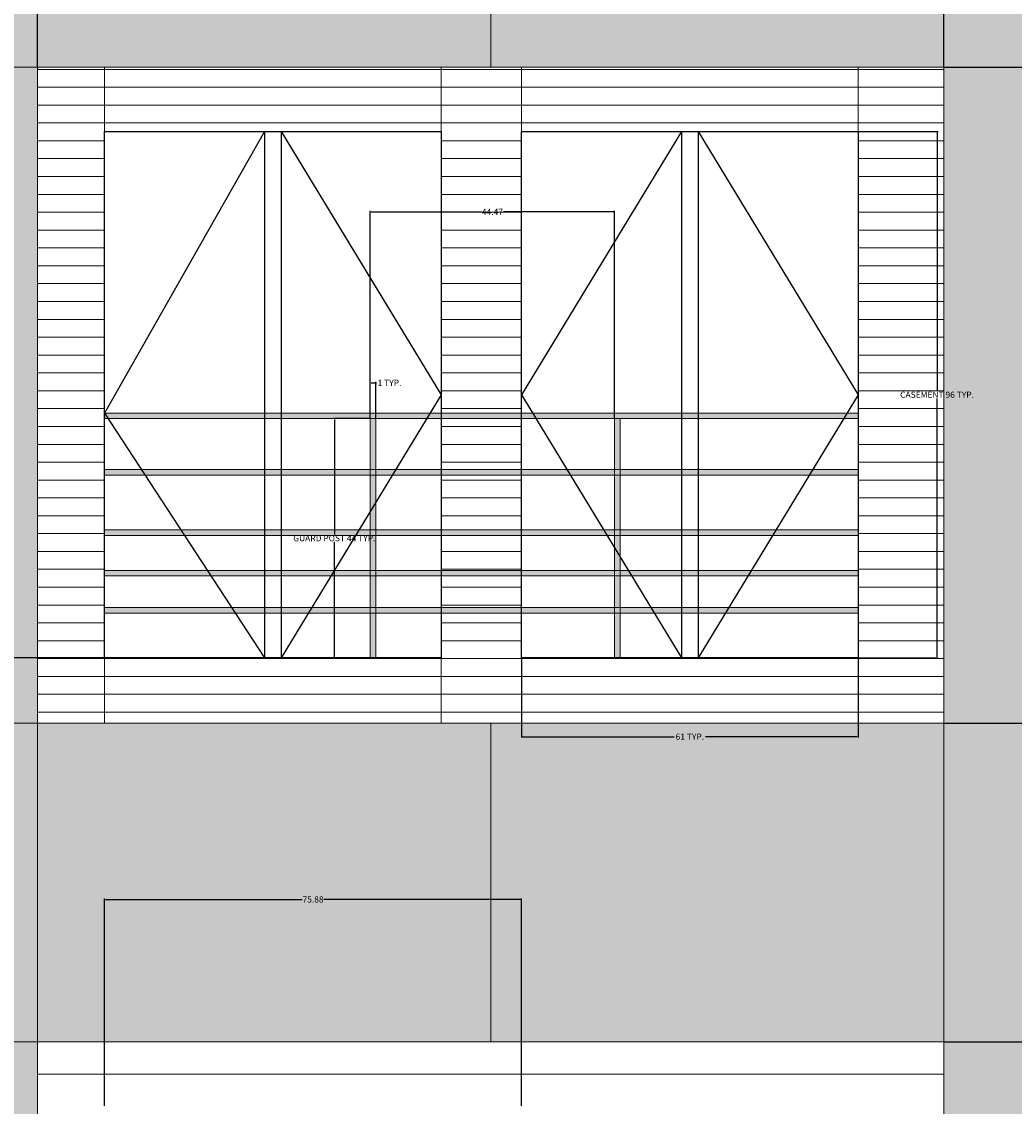
# Model space of a CAD drawing. Units: inches. Extents: x 8 to 634, y 41 to 867.
# Tile 6 of 21: x 117 to 297, y 380 to 577. Entities that reach past the tile are written whole.
import ezdxf

# ---------------------------------------------------------------- set-up
doc = ezdxf.new("R2010")
doc.units = ezdxf.units.IN
doc.header["$MEASUREMENT"] = 0
for name, color, linetype, lineweight in [('A-ANNO-DIMS', 2, 'Continuous', 18), ('A-FLOR-HRAL', 7, 'Continuous', 18), ('A-FLOR-HRAL-PATT', 252, 'Continuous', 9), ('A-GLAZ', 4, 'Continuous', 25), ('A-WALL-PANL', 7, 'Continuous', 18), ('A-WALL-PATT', 8, 'Continuous', 9)]:
    doc.layers.add(name, color=color, linetype=linetype, lineweight=lineweight)
doc.styles.get("Standard").update_dxf_attribs({"font": 'arial.ttf'})
doc.dimstyles.get("Standard").update_dxf_attribs({"dimtxt": 1.125, "dimasz": 0.18, "dimexe": 0.18, "dimexo": 0.0625, "dimgap": 0.09, "dimtad": 0, "dimtih": 1, "dimtoh": 1, "dimdec": 4, "dimzin": 0, "dimdsep": 46, "dimlunit": 4, "dimtxsty": 'Standard', "dimcen": 0.09, "dimadec": 0, "dimazin": 0, "dimtfac": 1, "dimtdec": 4, "dimtofl": 0, "dimtmove": 0, "dimatfit": 3, "dimfxl": 1, "dimtolj": 1, "dimtzin": 0, "dimarcsym": 0})

# ---------------------------------------------------------------- blocks, each defined once
blk = doc.blocks.new('WIN-CASEMENT-FRAME')
for p, q in [((29.12, 95.77), (29.12, 0)), ((32.12, 95.77), (32.12, 0))]:
    blk.add_line(p, q)
blk.add_lwpolyline([(0, 95.77), (61.23, 95.77), (61.23, 0), (0, 0)], close=True)
blk = doc.blocks.new('GUARD-POST')
for p, q in [((0, 42.52), (0, 43.52)), ((1, 42.52), (1, 43.52)), ((0, 42.52), (0, 0)), ((1, 42.52), (1, 0))]:
    blk.add_line(p, q)
blk = doc.blocks.new('*D13')
at = {"layer": 'A-ANNO-DIMS', "color": 0, "lineweight": -2, "transparency": 16777216}
for p, q in [((269.05, 557.42), (283.53, 557.42)), ((283.35, 557.24), (283.35, 510.21)), ((283.35, 461.83), (283.35, 508.86)), ((269.05, 461.65), (283.53, 461.65))]:
    blk.add_line(p, q, dxfattribs=at)
at = {"layer": 'A-ANNO-DIMS', "color": 0, "transparency": 16777216}
for points in [[(283.32, 557.24), (283.38, 557.24), (283.35, 557.42)], [(283.32, 461.83), (283.38, 461.83), (283.35, 461.65)]]:
    blk.add_solid(points, dxfattribs=at)
at = {"layer": 'Defpoints', "color": 0, "transparency": 16777216}
for p in [(268.99, 557.42), (283.35, 557.42), (268.99, 461.65)]:
    blk.add_point(p, dxfattribs=at)
at = {"layer": 'A-ANNO-DIMS', "color": 0, "transparency": 16777216, "insert": (283.35, 509.53), "char_height": 1.125, "attachment_point": 5}
blk.add_mtext('\\A1;CASEMENT 96 TYP.', dxfattribs=at)
blk = doc.blocks.new('*D14')
at = {"layer": 'A-ANNO-DIMS', "color": 0, "lineweight": -2, "transparency": 16777216}
for p, q in [((207.75, 461.59), (207.75, 447.11)), ((268.99, 461.59), (268.99, 447.11)), ((207.93, 447.29), (235.54, 447.29)), ((268.81, 447.29), (241.2, 447.29))]:
    blk.add_line(p, q, dxfattribs=at)
at = {"layer": 'A-ANNO-DIMS', "color": 0, "transparency": 16777216}
for points in [[(207.93, 447.32), (207.93, 447.26), (207.75, 447.29)], [(268.81, 447.32), (268.81, 447.26), (268.99, 447.29)]]:
    blk.add_solid(points, dxfattribs=at)
at = {"layer": 'Defpoints', "color": 0, "transparency": 16777216}
for p in [(207.75, 461.65), (268.99, 461.65), (268.99, 447.29)]:
    blk.add_point(p, dxfattribs=at)
at = {"layer": 'A-ANNO-DIMS', "color": 0, "transparency": 16777216, "insert": (238.37, 447.29), "char_height": 1.125, "attachment_point": 5}
blk.add_mtext('\\A1;61 TYP.', dxfattribs=at)
blk = doc.blocks.new('*D15')
at = {"layer": 'A-ANNO-DIMS', "color": 0, "lineweight": -2, "transparency": 16777216}
for p, q in [((180.15, 505.18), (173.51, 505.18)), ((173.69, 505), (173.69, 484.09)), ((173.69, 461.83), (173.69, 482.74)), ((180.15, 461.65), (173.51, 461.65))]:
    blk.add_line(p, q, dxfattribs=at)
at = {"layer": 'A-ANNO-DIMS', "color": 0, "transparency": 16777216}
for points in [[(173.66, 505), (173.72, 505), (173.69, 505.18)], [(173.66, 461.83), (173.72, 461.83), (173.69, 461.65)]]:
    blk.add_solid(points, dxfattribs=at)
at = {"layer": 'Defpoints', "color": 0, "transparency": 16777216}
for p in [(173.69, 505.18), (180.21, 505.18), (180.21, 461.65)]:
    blk.add_point(p, dxfattribs=at)
at = {"layer": 'A-ANNO-DIMS', "color": 0, "transparency": 16777216, "insert": (173.69, 483.41), "char_height": 1.125, "attachment_point": 5}
blk.add_mtext('\\A1;GUARD POST 44 TYP.', dxfattribs=at)
blk = doc.blocks.new('*D16')
at = {"layer": 'A-ANNO-DIMS', "color": 0, "lineweight": -2, "transparency": 16777216}
for p, q in [((180.21, 505.24), (180.21, 511.88)), ((180.39, 511.7), (181.03, 511.7)), ((181.21, 505.24), (181.21, 511.88)), ((181.21, 511.7), (181.39, 511.7))]:
    blk.add_line(p, q, dxfattribs=at)
at = {"layer": 'A-ANNO-DIMS', "color": 0, "transparency": 16777216}
for points in [[(180.39, 511.73), (180.39, 511.67), (180.21, 511.7)], [(181.03, 511.73), (181.03, 511.67), (181.21, 511.7)]]:
    blk.add_solid(points, dxfattribs=at)
at = {"layer": 'Defpoints', "color": 0, "transparency": 16777216}
for p in [(181.21, 511.7), (180.21, 505.18), (181.21, 505.18)]:
    blk.add_point(p, dxfattribs=at)
at = {"layer": 'A-ANNO-DIMS', "color": 0, "transparency": 16777216, "insert": (183.73, 511.7), "char_height": 1.125, "attachment_point": 5}
blk.add_mtext('\\A1;1 TYP.', dxfattribs=at)
blk = doc.blocks.new('*D20')
at = {"layer": 'A-ANNO-DIMS', "color": 0, "lineweight": -2, "transparency": 16777216}
for p, q in [((144.29, 828.98), (9.51, 828.98)), ((9.69, 828.8), (9.69, 454.93)), ((9.69, 79.74), (9.69, 453.6)), ((47.28, 79.56), (9.51, 79.56))]:
    blk.add_line(p, q, dxfattribs=at)
at = {"layer": 'A-ANNO-DIMS', "color": 0, "transparency": 16777216}
for points in [[(9.66, 828.8), (9.72, 828.8), (9.69, 828.98)], [(9.66, 79.74), (9.72, 79.74), (9.69, 79.56)]]:
    blk.add_solid(points, dxfattribs=at)
at = {"layer": 'Defpoints', "color": 0, "transparency": 16777216}
for p in [(9.69, 828.98), (144.36, 828.98), (47.34, 79.56)]:
    blk.add_point(p, dxfattribs=at)
at = {"layer": 'A-ANNO-DIMS', "color": 0, "transparency": 16777216, "insert": (9.69, 454.27), "char_height": 1.125, "attachment_point": 5}
blk.add_mtext('\\A1;749.4', dxfattribs=at)
blk = doc.blocks.new('*D41')
at = {"layer": 'A-ANNO-DIMS', "color": 0, "lineweight": -2, "transparency": 16777216}
for p, q in [((131.88, 380.07), (131.88, 417.84)), ((132.06, 417.66), (167.83, 417.66)), ((207.57, 417.66), (171.8, 417.66)), ((207.75, 380.07), (207.75, 417.84))]:
    blk.add_line(p, q, dxfattribs=at)
at = {"layer": 'A-ANNO-DIMS', "color": 0, "transparency": 16777216}
for points in [[(132.06, 417.69), (132.06, 417.63), (131.88, 417.66)], [(207.57, 417.69), (207.57, 417.63), (207.75, 417.66)]]:
    blk.add_solid(points, dxfattribs=at)
at = {"layer": 'Defpoints', "color": 0, "transparency": 16777216}
for p in [(207.75, 417.66), (131.88, 380.01), (207.75, 380.01)]:
    blk.add_point(p, dxfattribs=at)
at = {"layer": 'A-ANNO-DIMS', "color": 0, "transparency": 16777216, "insert": (169.82, 417.66), "char_height": 1.125, "attachment_point": 5}
blk.add_mtext('\\A1;75.88', dxfattribs=at)
blk = doc.blocks.new('*D43')
at = {"layer": 'A-ANNO-DIMS', "color": 0, "lineweight": -2, "transparency": 16777216}
for p, q in [((131.81, 461.65), (94.05, 461.65)), ((94.23, 461.47), (94.23, 373.6)), ((94.23, 284.42), (94.23, 372.29)), ((131.81, 284.24), (94.05, 284.24))]:
    blk.add_line(p, q, dxfattribs=at)
at = {"layer": 'A-ANNO-DIMS', "color": 0, "transparency": 16777216}
for points in [[(94.2, 461.47), (94.26, 461.47), (94.23, 461.65)], [(94.2, 284.42), (94.26, 284.42), (94.23, 284.24)]]:
    blk.add_solid(points, dxfattribs=at)
at = {"layer": 'Defpoints', "color": 0, "transparency": 16777216}
for p in [(94.23, 461.65), (131.88, 461.65), (131.88, 284.24)]:
    blk.add_point(p, dxfattribs=at)
at = {"layer": 'A-ANNO-DIMS', "color": 0, "transparency": 16777216, "insert": (94.23, 372.95), "char_height": 1.125, "attachment_point": 5}
blk.add_mtext('\\A1;177.4', dxfattribs=at)
blk = doc.blocks.new('*D57')
at = {"layer": 'A-ANNO-DIMS', "color": 0, "lineweight": -2, "transparency": 16777216}
for p, q in [((119.71, 569.23), (119.71, 607)), ((119.89, 606.82), (200.22, 606.82)), ((284.43, 606.82), (204.09, 606.82)), ((284.61, 569.23), (284.61, 607))]:
    blk.add_line(p, q, dxfattribs=at)
at = {"layer": 'A-ANNO-DIMS', "color": 0, "transparency": 16777216}
for points in [[(119.89, 606.85), (119.89, 606.79), (119.71, 606.82)], [(284.43, 606.85), (284.43, 606.79), (284.61, 606.82)]]:
    blk.add_solid(points, dxfattribs=at)
at = {"layer": 'Defpoints', "color": 0, "transparency": 16777216}
for p in [(284.61, 606.82), (119.71, 569.17), (284.61, 569.17)]:
    blk.add_point(p, dxfattribs=at)
at = {"layer": 'A-ANNO-DIMS', "color": 0, "transparency": 16777216, "insert": (202.16, 606.82), "char_height": 1.125, "attachment_point": 5}
blk.add_mtext('\\A1;164.9', dxfattribs=at)
blk = doc.blocks.new('*D58')
at = {"layer": 'A-ANNO-DIMS', "color": 0, "lineweight": -2, "transparency": 16777216}
for p, q in [((47.34, 569.23), (47.34, 607)), ((47.52, 606.82), (81.54, 606.82)), ((119.53, 606.82), (85.51, 606.82)), ((119.71, 569.23), (119.71, 607))]:
    blk.add_line(p, q, dxfattribs=at)
at = {"layer": 'A-ANNO-DIMS', "color": 0, "transparency": 16777216}
for points in [[(47.52, 606.85), (47.52, 606.79), (47.34, 606.82)], [(119.53, 606.85), (119.53, 606.79), (119.71, 606.82)]]:
    blk.add_solid(points, dxfattribs=at)
at = {"layer": 'Defpoints', "color": 0, "transparency": 16777216}
for p in [(119.71, 606.82), (47.34, 569.17), (119.71, 569.17)]:
    blk.add_point(p, dxfattribs=at)
at = {"layer": 'A-ANNO-DIMS', "color": 0, "transparency": 16777216, "insert": (83.52, 606.82), "char_height": 1.125, "attachment_point": 5}
blk.add_mtext('\\A1;72.37', dxfattribs=at)
blk = doc.blocks.new('*D59')
at = {"layer": 'A-ANNO-DIMS', "color": 0, "lineweight": -2, "transparency": 16777216}
for p, q in [((284.67, 449.75), (322.44, 449.75)), ((322.26, 449.57), (322.26, 421.42)), ((322.26, 391.94), (322.26, 420.09)), ((284.67, 391.76), (322.44, 391.76))]:
    blk.add_line(p, q, dxfattribs=at)
at = {"layer": 'A-ANNO-DIMS', "color": 0, "transparency": 16777216}
for points in [[(322.23, 449.57), (322.29, 449.57), (322.26, 449.75)], [(322.23, 391.94), (322.29, 391.94), (322.26, 391.76)]]:
    blk.add_solid(points, dxfattribs=at)
at = {"layer": 'Defpoints', "color": 0, "transparency": 16777216}
for p in [(284.61, 449.75), (284.61, 391.76), (322.26, 391.76)]:
    blk.add_point(p, dxfattribs=at)
at = {"layer": 'A-ANNO-DIMS', "color": 0, "transparency": 16777216, "insert": (322.26, 420.76), "char_height": 1.125, "attachment_point": 5}
blk.add_mtext('\\A1;57.99', dxfattribs=at)
blk = doc.blocks.new('*D60')
at = {"layer": 'A-ANNO-DIMS', "color": 0, "lineweight": -2, "transparency": 16777216}
for p, q in [((284.67, 569.17), (322.44, 569.17)), ((322.26, 568.99), (322.26, 510.13)), ((322.26, 449.93), (322.26, 508.8)), ((284.67, 449.75), (322.44, 449.75))]:
    blk.add_line(p, q, dxfattribs=at)
at = {"layer": 'A-ANNO-DIMS', "color": 0, "transparency": 16777216}
for points in [[(322.23, 568.99), (322.29, 568.99), (322.26, 569.17)], [(322.23, 449.93), (322.29, 449.93), (322.26, 449.75)]]:
    blk.add_solid(points, dxfattribs=at)
at = {"layer": 'Defpoints', "color": 0, "transparency": 16777216}
for p in [(284.61, 569.17), (284.61, 449.75), (322.26, 449.75)]:
    blk.add_point(p, dxfattribs=at)
at = {"layer": 'A-ANNO-DIMS', "color": 0, "transparency": 16777216, "insert": (322.26, 509.46), "char_height": 1.125, "attachment_point": 5}
blk.add_mtext('\\A1;119.42', dxfattribs=at)
blk = doc.blocks.new('*D62')
at = {"layer": 'A-ANNO-DIMS', "color": 0, "lineweight": -2, "transparency": 16777216}
for p, q in [((180.21, 505.24), (180.21, 543.01)), ((224.68, 505.24), (224.68, 543.01)), ((180.39, 542.83), (200.44, 542.83)), ((224.5, 542.83), (204.46, 542.83))]:
    blk.add_line(p, q, dxfattribs=at)
at = {"layer": 'A-ANNO-DIMS', "color": 0, "transparency": 16777216}
for points in [[(180.39, 542.86), (180.39, 542.8), (180.21, 542.83)], [(224.5, 542.86), (224.5, 542.8), (224.68, 542.83)]]:
    blk.add_solid(points, dxfattribs=at)
at = {"layer": 'Defpoints', "color": 0, "transparency": 16777216}
for p in [(224.68, 542.83), (180.21, 505.18), (224.68, 505.18)]:
    blk.add_point(p, dxfattribs=at)
at = {"layer": 'A-ANNO-DIMS', "color": 0, "transparency": 16777216, "insert": (202.45, 542.83), "char_height": 1.125, "attachment_point": 5}
blk.add_mtext('\\A1;44.47', dxfattribs=at)

msp = doc.modelspace()

# ---------------------------------------------------------------- hatches: boundary and pattern name
at = {"layer": 'A-FLOR-HRAL-PATT', "transparency": 33554681}
h = msp.add_hatch(color=256, dxfattribs=at)
h.dxf.hatch_style = 1
h.paths.add_polyline_path([(266.9465, 506.1755), (239.872, 506.1755), (239.872, 505.1755), (266.3384, 505.1755)])
h.paths.add_polyline_path([(236.872, 506.1755), (209.7974, 506.1755), (210.4055, 505.1755), (236.872, 505.1755)])
h.paths.add_polyline_path([(239.872, 506.1755), (236.872, 506.1755), (236.872, 505.1755), (239.872, 505.1755)])
h.paths.add_polyline_path([(268.9893, 506.1755), (266.9465, 506.1755), (266.3384, 505.1755), (268.9893, 505.1755)])
h.paths.add_polyline_path([(268.9893, 495.8921), (260.6935, 495.8921), (260.0854, 494.8921), (268.9893, 494.8921)])
h.paths.add_polyline_path([(260.6935, 495.8921), (239.872, 495.8921), (239.872, 494.8921), (260.0854, 494.8921)])
h.paths.add_polyline_path([(239.872, 495.8921), (236.872, 495.8921), (236.872, 494.8921), (239.872, 494.8921)])
h.paths.add_polyline_path([(236.872, 495.8921), (225.6812, 495.8921), (225.6812, 494.8921), (236.872, 494.8921)])
h.paths.add_polyline_path([(191.0689, 506.1755), (163.9944, 506.1755), (163.9944, 505.1755), (190.4608, 505.1755)])
h.paths.add_polyline_path([(193.1116, 506.1755), (191.0689, 506.1755), (190.4608, 505.1755), (193.1116, 505.1755)])
h.paths.add_polyline_path([(209.7974, 506.1755), (207.7547, 506.1755), (207.7547, 505.1755), (210.4055, 505.1755)])
h.paths.add_polyline_path([(207.7547, 506.1755), (193.1116, 506.1755), (193.1116, 505.1755), (207.7547, 505.1755)])
h.paths.add_polyline_path([(207.7547, 495.8921), (193.1116, 495.8921), (193.1116, 494.8921), (207.7547, 494.8921)])
h.paths.add_polyline_path([(216.0505, 495.8921), (207.7547, 495.8921), (207.7547, 494.8921), (216.6586, 494.8921)])
h.paths.add_polyline_path([(224.6812, 495.8921), (216.0505, 495.8921), (216.6586, 494.8921), (224.6812, 494.8921)])
h.paths.add_polyline_path([(225.6812, 495.8921), (224.6812, 495.8921), (224.6812, 494.8921), (225.6812, 494.8921)])
h.paths.add_polyline_path([(222.7266, 484.913), (207.7547, 484.913), (207.7547, 483.913), (223.3347, 483.913)])
h.paths.add_polyline_path([(207.7547, 484.913), (193.1116, 484.913), (193.1116, 483.913), (207.7547, 483.913)])
h.paths.add_polyline_path([(225.6812, 484.913), (224.6812, 484.913), (224.6812, 483.913), (225.6812, 483.913)])
h.paths.add_polyline_path([(224.6812, 484.913), (222.7266, 484.913), (223.3347, 483.913), (224.6812, 483.913)])
h.paths.add_polyline_path([(236.872, 484.913), (225.6812, 484.913), (225.6812, 483.913), (236.872, 483.913)])
h.paths.add_polyline_path([(239.872, 484.913), (236.872, 484.913), (236.872, 483.913), (239.872, 483.913)])
h.paths.add_polyline_path([(254.0173, 484.913), (239.872, 484.913), (239.872, 483.913), (253.4093, 483.913)])
h.paths.add_polyline_path([(268.9893, 484.913), (254.0173, 484.913), (253.4093, 483.913), (268.9893, 483.913)])
h.paths.add_polyline_path([(268.9893, 477.5606), (249.5465, 477.5606), (248.9384, 476.5606), (268.9893, 476.5606)])
h.paths.add_polyline_path([(249.5465, 477.5606), (239.872, 477.5606), (239.872, 476.5606), (248.9384, 476.5606)])
h.paths.add_polyline_path([(245.427, 470.7859), (239.872, 470.7859), (239.872, 469.7859), (244.8189, 469.7859)])
h.paths.add_polyline_path([(268.9893, 470.7859), (245.427, 470.7859), (244.8189, 469.7859), (268.9893, 469.7859)])
h.paths.add_polyline_path([(239.872, 470.7859), (236.872, 470.7859), (236.872, 469.7859), (239.872, 469.7859)])
h.paths.add_polyline_path([(239.872, 477.5606), (236.872, 477.5606), (236.872, 476.5606), (239.872, 476.5606)])
h.paths.add_polyline_path([(236.872, 477.5606), (227.1975, 477.5606), (227.8055, 476.5606), (236.872, 476.5606)])
h.paths.add_polyline_path([(236.872, 470.7859), (231.317, 470.7859), (231.9251, 469.7859), (236.872, 469.7859)])
h.paths.add_polyline_path([(231.317, 470.7859), (225.6812, 470.7859), (225.6812, 469.7859), (231.9251, 469.7859)])
h.paths.add_polyline_path([(225.6812, 470.7859), (224.6812, 470.7859), (224.6812, 469.7859), (225.6812, 469.7859)])
h.paths.add_polyline_path([(225.6812, 469.7859), (224.6812, 469.7859), (224.6812, 461.6505), (225.6812, 461.6505)])
h.paths.add_polyline_path([(225.6812, 476.5606), (224.6812, 476.5606), (224.6812, 470.7859), (225.6812, 470.7859)])
h.paths.add_polyline_path([(225.6812, 477.5606), (224.6812, 477.5606), (224.6812, 476.5606), (225.6812, 476.5606)])
h.paths.add_polyline_path([(225.6812, 480.0542), (224.6812, 481.6987), (224.6812, 477.5606), (225.6812, 477.5606)])
h.paths.add_polyline_path([(227.1975, 477.5606), (225.6812, 477.5606), (225.6812, 476.5606), (227.8055, 476.5606)])
h.paths.add_polyline_path([(224.6812, 477.5606), (207.7547, 477.5606), (207.7547, 476.5606), (224.6812, 476.5606)])
h.paths.add_polyline_path([(224.6812, 470.7859), (207.7547, 470.7859), (207.7547, 469.7859), (224.6812, 469.7859)])
h.paths.add_polyline_path([(225.6812, 483.913), (224.6812, 483.913), (224.6812, 481.6987), (225.6812, 480.0542)])
h.paths.add_polyline_path([(207.7547, 477.5606), (193.1116, 477.5606), (193.1116, 476.5606), (207.7547, 476.5606)])
h.paths.add_polyline_path([(207.7547, 470.7859), (193.1116, 470.7859), (193.1116, 469.7859), (207.7547, 469.7859)])
h.paths.add_polyline_path([(193.1116, 470.7859), (181.2144, 470.7859), (181.2144, 469.7859), (193.1116, 469.7859)])
h.paths.add_polyline_path([(193.1116, 477.5606), (181.2144, 477.5606), (181.2144, 476.5606), (193.1116, 476.5606)])
h.paths.add_polyline_path([(181.2144, 470.7859), (131.8771, 470.7859), (131.8771, 469.7859), (181.2144, 469.7859)])
h = msp.add_hatch(color=256, dxfattribs=at)
h.dxf.hatch_style = 1
h.paths.add_polyline_path([(180.2144, 477.5606), (173.6689, 477.5606), (173.0608, 476.5606), (180.2144, 476.5606)])
h.paths.add_polyline_path([(181.2144, 483.913), (180.2144, 483.913), (180.2144, 477.5606), (181.2144, 477.5606)])
h.paths.add_polyline_path([(181.2144, 476.5606), (180.2144, 476.5606), (180.2144, 470.7859), (181.2144, 470.7859)])
h.paths.add_polyline_path([(181.2144, 477.5606), (180.2144, 477.5606), (180.2144, 476.5606), (181.2144, 476.5606)])
h.paths.add_polyline_path([(181.2144, 469.7859), (180.2144, 469.7859), (180.2144, 461.6505), (181.2144, 461.6505)])
h.paths.add_polyline_path([(163.9944, 477.5606), (160.9944, 477.5606), (160.9944, 476.5606), (163.9944, 476.5606)])
h.paths.add_polyline_path([(173.6689, 477.5606), (163.9944, 477.5606), (163.9944, 476.5606), (173.0608, 476.5606)])
h.paths.add_polyline_path([(160.9944, 477.5606), (150.5899, 477.5606), (151.2439, 476.5606), (160.9944, 476.5606)])
h.paths.add_polyline_path([(150.5899, 477.5606), (131.8771, 477.5606), (131.8771, 476.5606), (151.2439, 476.5606)])
h.paths.add_polyline_path([(160.9944, 484.913), (145.7818, 484.913), (146.4357, 483.913), (160.9944, 483.913)])
h.paths.add_polyline_path([(145.7818, 484.913), (131.8771, 484.913), (131.8771, 483.913), (146.4357, 483.913)])
h.paths.add_polyline_path([(163.9944, 484.913), (160.9944, 484.913), (160.9944, 483.913), (163.9944, 483.913)])
h.paths.add_polyline_path([(178.1397, 484.913), (163.9944, 484.913), (163.9944, 483.913), (177.5316, 483.913)])
h.paths.add_polyline_path([(181.2144, 484.913), (180.2144, 484.913), (180.2144, 483.913), (181.2144, 483.913)])
h.paths.add_polyline_path([(181.2144, 489.9695), (180.2144, 488.3249), (180.2144, 484.913), (181.2144, 484.913)])
h.paths.add_polyline_path([(193.1116, 484.913), (181.2144, 484.913), (181.2144, 483.913), (193.1116, 483.913)])
h.paths.add_polyline_path([(180.2144, 484.913), (178.1397, 484.913), (177.5316, 483.913), (180.2144, 483.913)])
h.paths.add_polyline_path([(181.2144, 495.8921), (180.2144, 495.8921), (180.2144, 494.8921), (181.2144, 494.8921)])
h.paths.add_polyline_path([(181.2144, 494.8921), (180.2144, 494.8921), (180.2144, 488.3249), (181.2144, 489.9695)])
h.paths.add_polyline_path([(184.8158, 495.8921), (181.2144, 495.8921), (181.2144, 494.8921), (184.2078, 494.8921)])
h.paths.add_polyline_path([(193.1116, 495.8921), (184.8158, 495.8921), (184.2078, 494.8921), (193.1116, 494.8921)])
h.paths.add_polyline_path([(180.2144, 495.8921), (163.9944, 495.8921), (163.9944, 494.8921), (180.2144, 494.8921)])
h.paths.add_polyline_path([(163.9944, 495.8921), (160.9944, 495.8921), (160.9944, 494.8921), (163.9944, 494.8921)])
h.paths.add_polyline_path([(160.9944, 495.8921), (138.6019, 495.8921), (139.2559, 494.8921), (160.9944, 494.8921)])
h.paths.add_polyline_path([(138.6019, 495.8921), (131.8771, 495.8921), (131.8771, 494.8921), (139.2559, 494.8921)])
h.paths.add_polyline_path([(181.2144, 504.1755), (181.2144, 505.1755), (180.2144, 505.1755), (180.2144, 504.1755), (180.2144, 495.8921), (181.2144, 495.8921)])
h.paths.add_polyline_path([(225.6812, 494.8921), (224.6812, 494.8921), (224.6812, 484.913), (225.6812, 484.913)])
h.paths.add_polyline_path([(225.6812, 495.8921), (224.6812, 495.8921), (224.6812, 494.8921), (225.6812, 494.8921)])
h.paths.add_polyline_path([(225.6812, 504.1755), (225.6812, 505.1755), (224.6812, 505.1755), (224.6812, 504.1755), (224.6812, 495.8921), (225.6812, 495.8921)])
h.paths.add_polyline_path([(131.8771, 506.1755), (131.8771, 505.1755), (132.531, 505.1755)], flags=17)
h.paths.add_polyline_path([(193.1116, 506.1755), (131.8771, 506.1755), (132.531, 505.1755), (193.1116, 505.1755)])
at = {"layer": 'A-WALL-PATT', "transparency": 33554687}
h = msp.add_hatch(dxfattribs=at)
h.set_pattern_fill('AR-CONC', color=256, scale=3.2)
h.paths.add_polyline_path([(119.7065, 697.6655), (47.3401, 697.6655), (47.3401, 569.1705), (119.7065, 569.1705)])
h.paths.add_polyline_path([(202.1558, 697.6655), (119.7065, 697.6655), (119.7065, 569.1705), (202.1558, 569.1705)])
h.paths.add_polyline_path([(284.6051, 697.6655), (202.1558, 697.6655), (202.1558, 569.1705), (284.6051, 569.1705)])
h.paths.add_polyline_path([(119.7065, 569.1705), (47.3401, 569.1705), (47.3401, 523.5555), (47.3401, 449.7533), (119.7065, 449.7533)])
h.paths.add_polyline_path([(342.6544, 682.1444), (360.785, 697.6655), (284.6051, 697.6655), (284.6051, 569.1705), (342.6544, 569.1705)])
h.paths.add_polyline_path([(342.6544, 569.1705), (284.6051, 569.1705), (284.6051, 449.7533), (342.6544, 449.7533)])
h.paths.add_polyline_path([(418.2881, 691.978), (418.2881, 697.6655), (360.785, 697.6655), (360.785, 569.1705), (418.2881, 569.1705)])
h.paths.add_polyline_path([(418.2881, 569.1705), (360.785, 569.1705), (360.785, 523.5555), (360.785, 449.7533), (418.2881, 449.7533)])
h.paths.add_polyline_path([(594.3501, 697.6655), (539.0002, 697.6655), (539.0002, 691.978), (539.0002, 569.1705), (594.3501, 569.1705)])
h.paths.add_polyline_path([(594.3501, 523.5555), (594.3501, 569.1705), (539.0002, 569.1705), (539.0002, 451.6305), (594.3501, 451.6305)])
h.paths.add_polyline_path([(594.3501, 451.6305), (539.0002, 451.6305), (539.0002, 391.7598), (594.3501, 391.7598)])
h.paths.add_polyline_path([(594.3501, 391.7598), (539.0002, 391.7598), (539.0002, 276.166), (594.3501, 276.166)])
h.paths.add_polyline_path([(418.2881, 449.7533), (360.785, 449.7533), (360.785, 391.7598), (418.2881, 391.7598)])
h.paths.add_polyline_path([(342.6544, 449.7533), (284.6051, 449.7533), (284.6051, 391.7598), (342.6544, 391.7598)])
h.paths.add_polyline_path([(342.6544, 391.7598), (284.6051, 391.7598), (284.6051, 272.3426), (342.6544, 272.3426)])
h.paths.add_polyline_path([(418.2881, 391.7598), (360.785, 391.7598), (360.785, 272.3426), (418.2881, 272.3426)])
h.paths.add_polyline_path([(418.2881, 272.3426), (360.785, 272.3426), (360.785, 235.5555), (418.2881, 235.5555)])
h.paths.add_polyline_path([(342.6544, 272.3426), (284.6051, 272.3426), (284.6051, 235.5555), (295.0049, 235.5555), (342.6544, 235.5555)])
h.paths.add_polyline_path([(594.3501, 276.166), (539.0002, 276.166), (539.0002, 228.4951), (594.3501, 228.4951)])
h.paths.add_polyline_path([(594.3501, 228.4951), (539.0002, 228.4951), (539.0002, 91.5417), (594.3501, 91.5417)])
h.paths.add_polyline_path([(418.2881, 235.5555), (360.785, 235.5555), (360.785, 91.5417), (418.2881, 91.5417)])
h.paths.add_polyline_path([(284.6051, 272.3426), (119.7065, 272.3426), (119.7065, 235.5555), (284.6051, 235.5555)])
h.paths.add_polyline_path([(119.7065, 272.3426), (47.3401, 272.3426), (47.3401, 235.5555), (47.3401, 91.5555), (63.5448, 91.5555), (63.5448, 227.8036), (268.998, 227.8036), (268.998, 91.5555), (295.0049, 91.5555), (295.0049, 222.583), (271.9787, 222.583), (271.9787, 229.0481), (62.4019, 229.0481), (62.4019, 222.583), (61.1827, 222.583), (61.1827, 235.5555), (119.7065, 235.5555)])
h.paths.add_polyline_path([(119.7065, 391.7598), (47.3401, 391.7598), (47.3401, 379.5555), (47.3401, 272.3426), (119.7065, 272.3426)])
h.paths.add_polyline_path([(119.7065, 449.7533), (47.3401, 449.7533), (47.3401, 391.7598), (119.7065, 391.7598)])
h.paths.add_polyline_path([(202.1558, 449.7533), (119.7065, 449.7533), (119.7065, 391.7598), (202.1558, 391.7598)])
h.paths.add_polyline_path([(284.6051, 449.7533), (202.1558, 449.7533), (202.1558, 391.7598), (284.6051, 391.7598)])
at = {"layer": 'A-WALL-PATT', "transparency": 33554681}
h = msp.add_hatch(dxfattribs=at)
h.set_pattern_fill('ANSI31', color=256, scale=26, angle=135)
h.paths.add_polyline_path([(284.6051, 569.1705), (268.9893, 569.1705), (268.9893, 557.4192), (268.9893, 461.6505), (268.9893, 449.7533), (284.6051, 449.7533)])
h.paths.add_polyline_path([(207.7547, 557.4192), (207.7547, 569.1705), (193.1116, 569.1705), (193.1116, 557.4192), (193.1116, 506.1755), (207.7547, 506.1755)])
h.paths.add_polyline_path([(268.9893, 569.1705), (207.7547, 569.1705), (207.7547, 557.4192), (268.9893, 557.4192)])
h.paths.add_polyline_path([(193.1116, 569.1705), (131.8771, 569.1705), (131.8771, 557.4192), (193.1116, 557.4192)])
h.paths.add_polyline_path([(131.8771, 557.4192), (131.8771, 569.1705), (119.7065, 569.1705), (119.7065, 449.7533), (131.8771, 449.7533), (131.8771, 461.6505)])
h.paths.add_polyline_path([(193.1116, 461.6505), (131.8771, 461.6505), (131.8771, 449.7533), (193.1116, 449.7533)])
h.paths.add_polyline_path([(207.7547, 461.6505), (207.7547, 469.7859), (193.1116, 469.7859), (193.1116, 461.6505), (193.1116, 449.7533), (207.7547, 449.7533)])
h.paths.add_polyline_path([(268.9893, 461.6505), (207.7547, 461.6505), (207.7547, 449.7533), (268.9893, 449.7533)])
h.paths.add_polyline_path([(207.7547, 476.5606), (193.1116, 476.5606), (193.1116, 470.7859), (207.7547, 470.7859)])
h.paths.add_polyline_path([(207.7547, 483.913), (193.1116, 483.913), (193.1116, 477.5606), (207.7547, 477.5606)])
h.paths.add_polyline_path([(207.7547, 494.8921), (193.1116, 494.8921), (193.1116, 484.913), (207.7547, 484.913)])
h.paths.add_polyline_path([(207.7547, 505.1755), (193.1116, 505.1755), (193.1116, 495.8921), (207.7547, 495.8921)])
h = msp.add_hatch(dxfattribs=at)
h.set_pattern_fill('ANSI31', color=256, scale=63, angle=135)
h.paths.add_polyline_path([(284.6051, 391.7598), (119.7065, 391.7598), (119.7065, 272.3426), (284.6051, 272.3426)])
h.paths.add_polyline_path([(193.1116, 284.2398), (131.8771, 284.2398), (131.8771, 380.0085), (193.1116, 380.0085)], flags=16)
h.paths.add_polyline_path([(207.7547, 380.0085), (268.9893, 380.0085), (268.9893, 284.2398), (207.7547, 284.2398)], flags=16)
h.paths.add_polyline_path([(342.6544, 235.5555), (295.0049, 235.5555), (295.0049, 91.5417), (342.6544, 91.5417)])

# ---------------------------------------------------------------- linework, layer by layer
at = {"layer": 'A-FLOR-HRAL'}
for p, q in [((131.8771, 506.1755), (268.9893, 506.1755)), ((131.8771, 505.1755), (268.9893, 505.1755)), ((131.8771, 495.8921), (268.9893, 495.8921)), ((131.8771, 494.8921), (268.9893, 494.8921)), ((131.8771, 484.913), (268.9893, 484.913)), ((131.8771, 483.913), (268.9893, 483.913)), ((131.8771, 477.5606), (268.9893, 477.5606)), ((131.8771, 476.5606), (268.9893, 476.5606)), ((131.8771, 470.7859), (268.9893, 470.7859)), ((131.8771, 469.7859), (268.9893, 469.7859))]:
    msp.add_line(p, q, dxfattribs=at)
at = {"layer": 'A-GLAZ'}
for p, q in [((160.9944, 557.4192), (131.8771, 506.1755)), ((163.9944, 557.4192), (193.1116, 509.5348)), ((236.872, 557.4192), (207.7547, 509.5348)), ((239.872, 557.4192), (268.9893, 509.5348)), ((193.1116, 509.5348), (163.9944, 461.6505)), ((207.7547, 509.5348), (236.872, 461.6505)), ((268.9893, 509.5348), (239.872, 461.6505)), ((131.8771, 506.1755), (160.9944, 461.6505))]:
    msp.add_line(p, q, dxfattribs=at)
at = {"layer": 'A-WALL-PANL'}
for p, q in [((119.7065, 569.1705), (119.7065, 697.6655)), ((202.1558, 569.1705), (202.1558, 697.6655)), ((284.6051, 569.1705), (284.6051, 697.6655)), ((418.2881, 569.1705), (47.3401, 569.1705)), ((131.8771, 557.4192), (131.8771, 569.1705)), ((193.1116, 557.4192), (193.1116, 569.1705)), ((207.7547, 557.4192), (207.7547, 569.1705)), ((268.9893, 557.4192), (268.9893, 569.1705)), ((131.8771, 461.6505), (131.8771, 449.7533)), ((193.1116, 461.6505), (193.1116, 449.7533)), ((207.7547, 461.6505), (207.7547, 449.7533)), ((268.9893, 461.6505), (268.9893, 449.7533)), ((119.7065, 449.7533), (47.3401, 449.7533)), ((119.7065, 449.7533), (119.7065, 391.7598)), ((202.1558, 449.7533), (202.1558, 391.7598)), ((284.6051, 449.7533), (418.2881, 449.7533)), ((284.6051, 449.7533), (284.6051, 391.7598)), ((418.2881, 391.7598), (47.3401, 391.7598))]:
    msp.add_line(p, q, dxfattribs=at)
for points in [[(119.7065, 569.1705), (284.6051, 569.1705), (284.6051, 449.7533), (119.7065, 449.7533)], [(119.7065, 391.7598), (284.6051, 391.7598), (284.6051, 272.3426), (119.7065, 272.3426)]]:
    msp.add_lwpolyline(points, close=True, dxfattribs=at)

# ---------------------------------------------------------------- block references
at = {"layer": 'A-FLOR-HRAL'}
for p in [(180.214, 461.651), (224.6807, 461.651)]:
    msp.add_blockref('GUARD-POST', p, dxfattribs=at)
at = {"layer": 'A-GLAZ'}
for p in [(131.877, 461.651), (207.7546, 461.651)]:
    msp.add_blockref('WIN-CASEMENT-FRAME', p, dxfattribs=at)

# ---------------------------------------------------------------- dimensions: what is measured, and where the dimension line sits
at = {"layer": 'A-ANNO-DIMS'}
for base, p1, p2, angle, override, picture, middle in [((9.6901, 828.9821), (47.3401, 79.5555), (144.3564, 828.9821), 90, {"dimdec": 1, "dimlfac": 1, "dimrnd": 0, "dimzin": 0, "dimdsep": 46, "dimlunit": 2}, '*D20', (9.6901, 454.2688)), ((322.2551, 449.7533), (284.6051, 569.1705), (284.6051, 449.7533), 270, {"dimdec": 2, "dimlfac": 1, "dimrnd": 0, "dimzin": 0, "dimdsep": 46, "dimlunit": 2}, '*D60', (322.2551, 509.4619)), ((94.2271, 461.6505), (131.8771, 284.2398), (131.8771, 461.6505), 90, {"dimdec": 1, "dimlfac": 1, "dimrnd": 0, "dimzin": 0, "dimdsep": 46, "dimlunit": 2}, '*D43', (94.2271, 372.9452)), ((322.2551, 391.7598), (284.6051, 449.7533), (284.6051, 391.7598), 270, {"dimdec": 2, "dimlfac": 1, "dimrnd": 0, "dimzin": 0, "dimdsep": 46, "dimlunit": 2}, '*D59', (322.2551, 420.7566))]:
    dim = msp.add_linear_dim(base=base, p1=p1, p2=p2, angle=angle, dimstyle='Standard', override=override, dxfattribs=at)
    dim.commit()
    dim.dimension.update_dxf_attribs({"geometry": picture, "text_midpoint": middle})
for base, p1, p2, override, picture, middle in [((119.7065, 606.8205), (47.3401, 569.1705), (119.7065, 569.1705), {"dimdec": 2, "dimlfac": 1, "dimrnd": 0, "dimzin": 0, "dimdsep": 46, "dimlunit": 2}, '*D58', (83.5233, 606.8205)), ((284.6051, 606.8205), (119.7065, 569.1705), (284.6051, 569.1705), {"dimdec": 1, "dimlfac": 1, "dimrnd": 0, "dimzin": 0, "dimdsep": 46, "dimlunit": 2}, '*D57', (202.1558, 606.8205)), ((224.6812, 542.8255), (180.2144, 505.1755), (224.6812, 505.1755), {"dimdec": 2, "dimlfac": 1, "dimrnd": 0, "dimzin": 0, "dimdsep": 46, "dimlunit": 2}, '*D62', (202.4478, 542.8255)), ((207.7547, 417.6585), (131.8771, 380.0085), (207.7547, 380.0085), {"dimdec": 2, "dimlfac": 1, "dimrnd": 0, "dimzin": 0, "dimdsep": 46, "dimlunit": 2}, '*D41', (169.8159, 417.6585))]:
    dim = msp.add_linear_dim(base=base, p1=p1, p2=p2, dimstyle='Standard', override=override, dxfattribs=at)
    dim.commit()
    dim.dimension.update_dxf_attribs({"geometry": picture, "text_midpoint": middle})
for base, p1, p2, text, picture, middle in [((283.3546, 557.4192), (268.9893, 461.6505), (268.9893, 557.4192), 'CASEMENT <> TYP.', '*D13', (283.3546, 509.5348)), ((173.6857, 505.1755), (180.2144, 461.6505), (180.2144, 505.1755), 'GUARD POST <> TYP.', '*D15', (173.6857, 483.413))]:
    dim = msp.add_linear_dim(base=base, p1=p1, p2=p2, angle=90, text=text, dimstyle='Standard', override={"dimdec": 0, "dimlfac": 1, "dimrnd": 0, "dimzin": 0, "dimdsep": 46, "dimlunit": 2}, dxfattribs=at)
    dim.commit()
    dim.dimension.update_dxf_attribs({"geometry": picture, "text_midpoint": middle})
for base, p1, p2, picture, middle in [((181.2144, 511.7042), (180.2144, 505.1755), (181.2144, 505.1755), '*D16', (183.7325, 511.7042)), ((268.9893, 447.2852), (207.7547, 461.6505), (268.9893, 461.6505), '*D14', (238.372, 447.2852))]:
    dim = msp.add_linear_dim(base=base, p1=p1, p2=p2, text='<> TYP.', dimstyle='Standard', override={"dimdec": 0, "dimlfac": 1, "dimrnd": 0, "dimzin": 0, "dimdsep": 46, "dimlunit": 2}, dxfattribs=at)
    dim.commit()
    dim.dimension.update_dxf_attribs({"geometry": picture, "text_midpoint": middle})

doc.saveas('drawing.dxf')
